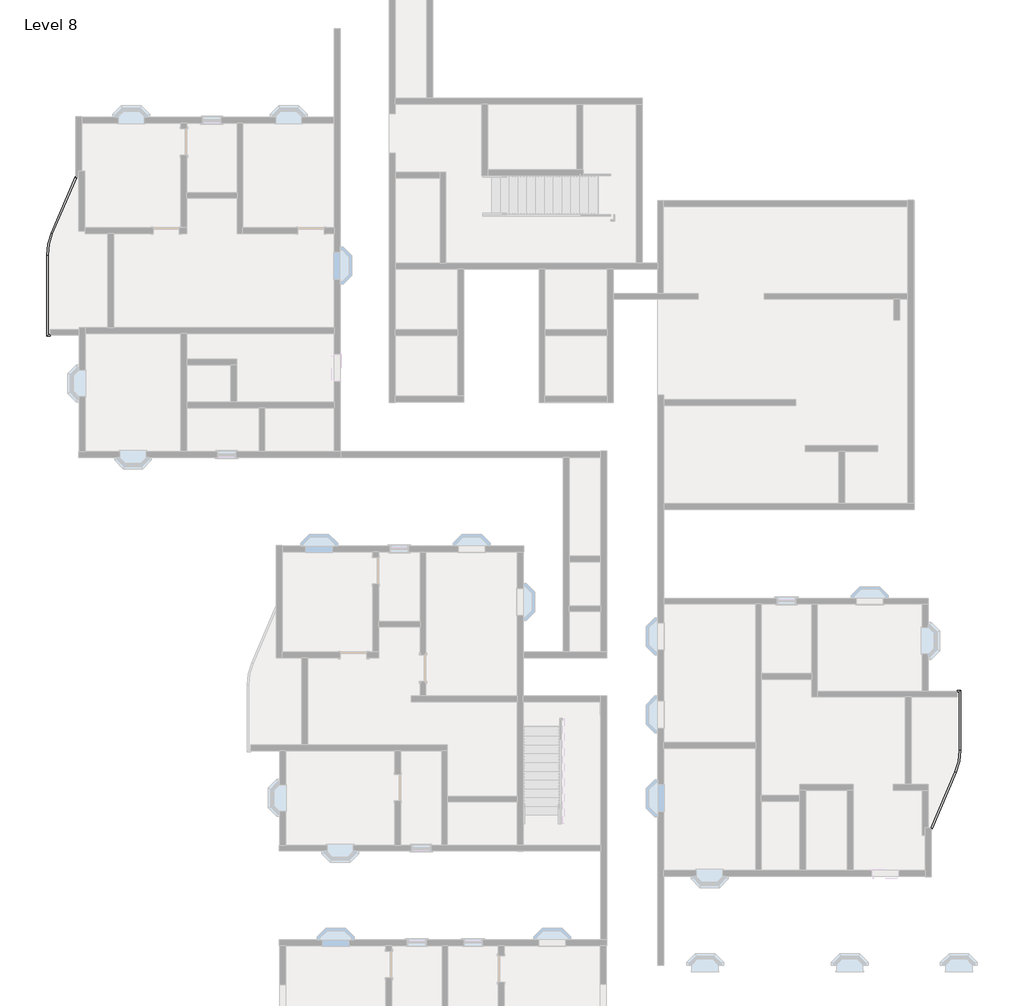
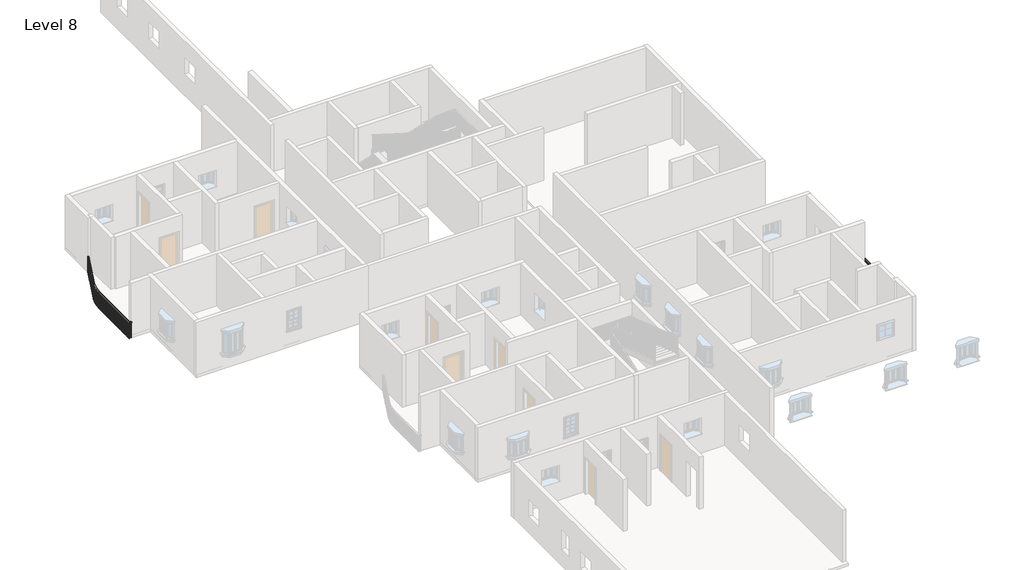
# One storey, part 9 of 14: 2 railings.
"""IFC4 building model written with IfcOpenShell, lengths in millimetres."""

from ifc_helpers import new_model, si_unit, frame, origin, place, context, project, spatial, polyline, circle_curve, outline, extrude, element, save
from ifc_brep_helpers import plane_surface, cylinder_surface, revolved_surface, advanced_brep

model = new_model("IFC4")

# Units and contexts
model_context = context("Model", 3, world=origin())
ifc_project = project(units=[si_unit("LENGTHUNIT", "METRE", prefix="MILLI")], contexts=[model_context])

# Site, building, storey
site = spatial("IfcSite", under=ifc_project)
building = spatial("IfcBuilding", under=site)
storey = spatial("IfcBuildingStorey", under=building, Name="Level 8", Elevation=21336.0)

# Railings
placement = place(None, origin())
element("IfcRailing", 1, ObjectType="Handrail - Rectangular", at=placement, inside=storey, context=model_context, shape_type="SolidModel", body=[
    advanced_brep(
    [(-19327.739878, 12446.0257339, 22250.4), (-19327.739878, 12446.0257339, 22199.6), (-19374.4383922, 12466.022953, 22199.6), (-19374.4383922, 12466.022953, 22250.4), (-20162.483418, 10496.6905323, 22250.4), (-20162.483418, 10496.6905323, 22199.6), (-20209.1819322, 10516.6877514, 22199.6), (-20209.1819322, 10516.6877514, 22250.4), (-20316.2891351, 9746.7948172, 22199.6), (-20316.2891351, 9746.7948172, 22250.4), (-20367.0891351, 9746.7948172, 22199.6), (-20367.0891351, 9746.7948172, 22250.4), (-20316.2891351, 7005.2583494, 22250.4), (-20316.2891351, 7005.2583494, 22199.6), (-20367.0891351, 6954.4583494, 22199.6), (-20367.0891351, 6954.4583494, 22250.4), (-20240.0891351, 7005.2583494, 22250.4), (-20240.0891351, 6954.4583494, 22250.4), (-20240.0891351, 6954.4583494, 22199.6), (-20240.0891351, 7005.2583494, 22199.6)],
    [
        (0, 1),
        (1, 2),
        (2, 3),
        (3, 0),
        (0, 4),
        (4, 5),
        (5, 1),
        (5, 6),
        (6, 2),
        (6, 7),
        (7, 3),
        (7, 4),
        (8, 5, circle_curve(frame((-18411.2891351, 9746.7948172, 22199.6), z_axis=(0.0, 0.0, -1.0), x_axis=(-0.919262090762392, 0.3936460446735823, 0.0)), 1905.0)),
        (4, 9, circle_curve(frame((-18411.2891351, 9746.7948172, 22250.4), z_axis=(0.0, 0.0, 1.0), x_axis=(-0.919262090762392, 0.3936460446735823, 0.0)), 1905.0)),
        (9, 8),
        (10, 6, circle_curve(frame((-18411.2891351, 9746.7948172, 22199.6), z_axis=(0.0, 0.0, -1.0), x_axis=(-0.919262090762392, 0.3936460446735823, 0.0)), 1955.8)),
        (8, 10),
        (11, 7, circle_curve(frame((-18411.2891351, 9746.7948172, 22250.4), z_axis=(0.0, 0.0, -1.0), x_axis=(-0.919262090762392, 0.3936460446735823, 0.0)), 1955.8)),
        (10, 11),
        (11, 9),
        (9, 12),
        (12, 13),
        (13, 8),
        (13, 14),
        (14, 10),
        (14, 15),
        (15, 11),
        (15, 12),
        (16, 17),
        (17, 18),
        (18, 19),
        (19, 16),
        (12, 16),
        (19, 13),
        (18, 14),
        (17, 15),
    ],
    [
        plane_surface(frame((-19351.0891351, 12456.0243434, 22250.4), z_axis=(0.3936460446735829, 0.9192620907623917, 0.0), x_axis=(0.9192620907623917, -0.3936460446735829, 0.0))),
        plane_surface(frame((-19327.739878, 12446.0257339, 22250.4), z_axis=(0.9192620907623916, -0.393646044673583, 0.0), x_axis=(-0.393646044673583, -0.9192620907623916, 0.0))),
        plane_surface(frame((-19327.739878, 12446.0257339, 22199.6), z_axis=(0.0, 0.0, -1.0), x_axis=(-0.393646044673583, -0.9192620907623916, 0.0))),
        plane_surface(frame((-19374.4383922, 12466.022953, 22199.6), z_axis=(-0.9192620907623917, 0.3936460446735826, 0.0), x_axis=(-0.3936460446735826, -0.9192620907623917, 0.0))),
        plane_surface(frame((-19374.4383922, 12466.022953, 22250.4), z_axis=(0.0, 0.0, 1.0), x_axis=(-0.3936460446735826, -0.9192620907623917, 0.0))),
        revolved_surface(polyline([(-20162.483418002357, 10496.690532303173, 22250.4), (-20162.483418002357, 10496.690532303173, 22199.6)]), (-18411.2891351, 9746.7948172, 22250.4), (0.0, 0.0, 1.0)),
        plane_surface(frame((-18411.2891351, 9746.7948172, 22199.6), z_axis=(0.0, 0.0, -1.0), x_axis=(-0.919262090762392, 0.3936460446735823, 0.0))),
        cylinder_surface(frame((-18411.2891351, 9746.7948172, 22250.4), z_axis=(0.0, 0.0, 1.0), x_axis=(-0.919262090762392, 0.3936460446735823, 0.0)), 1955.8),
        plane_surface(frame((-18411.2891351, 9746.7948172, 22250.4), z_axis=(0.0, 0.0, 1.0), x_axis=(-0.919262090762392, 0.3936460446735823, 0.0))),
        plane_surface(frame((-20316.2891351, 9746.7948172, 22250.4), z_axis=(1.0, 0.0, 0.0), x_axis=(0.0, -1.0, 0.0))),
        plane_surface(frame((-20316.2891351, 9746.7948172, 22199.6), z_axis=(0.0, 0.0, -1.0), x_axis=(0.0, -1.0, 0.0))),
        plane_surface(frame((-20367.0891351, 9746.7948172, 22199.6), z_axis=(-1.0, 0.0, 0.0), x_axis=(0.0, -1.0, 0.0))),
        plane_surface(frame((-20367.0891351, 9746.7948172, 22250.4), z_axis=(0.0, 0.0, 1.0), x_axis=(0.0, -1.0, 0.0))),
        plane_surface(frame((-20240.0891351, 6979.8583494, 22250.4), z_axis=(1.0, 0.0, 0.0), x_axis=(0.0, 1.0, 0.0))),
        plane_surface(frame((-20316.2891351, 7005.2583494, 22250.4), z_axis=(0.0, 1.0, 0.0), x_axis=(1.0, 0.0, 0.0))),
        plane_surface(frame((-20316.2891351, 7005.2583494, 22199.6), z_axis=(0.0, 0.0, -1.0), x_axis=(1.0, 0.0, 0.0))),
        plane_surface(frame((-20367.0891351, 6954.4583494, 22199.6), z_axis=(0.0, -1.0, 0.0), x_axis=(1.0, 0.0, 0.0))),
        plane_surface(frame((-20367.0891351, 6954.4583494, 22250.4), z_axis=(0.0, 0.0, 1.0), x_axis=(1.0, 0.0, 0.0))),
    ],
    [
        (0, [[1, 2, 3, 4]]),
        (1, [[-1, 5, 6, 7]]),
        (2, [[-2, -7, 8, 9]]),
        (3, [[-3, -9, 10, 11]]),
        (4, [[-4, -11, 12, -5]]),
        (5, [[13, -6, 14, 15]]),
        (6, [[16, -8, -13, 17]]),
        (7, [[18, -10, -16, 19]]),
        (8, [[-14, -12, -18, 20]]),
        (9, [[-15, 21, 22, 23]]),
        (10, [[-17, -23, 24, 25]]),
        (11, [[-19, -25, 26, 27]]),
        (12, [[-20, -27, 28, -21]]),
        (13, [[29, 30, 31, 32]]),
        (14, [[-22, 33, -32, 34]]),
        (15, [[-24, -34, -31, 35]]),
        (16, [[-26, -35, -30, 36]]),
        (17, [[-28, -36, -29, -33]]),
    ],
),
    extrude(outline(polyline([(-20351.2141351, 7013.1198172), (-20332.1641351, 7013.1198172), (-20332.1641351, 6994.0698172), (-20351.2141351, 6994.0698172), (-20351.2141351, 7013.1198172)])), frame((0.0, 0.0, 21336.0), z_axis=(0.0, 0.0, 1.0), x_axis=(1.0, 0.0, 0.0)), (0.0, 0.0, 1.0), 863.6),
    extrude(outline(polyline([(-20351.2141351, 7114.7198172), (-20332.1641351, 7114.7198172), (-20332.1641351, 7095.6698172), (-20351.2141351, 7095.6698172), (-20351.2141351, 7114.7198172)])), frame((0.0, 0.0, 21336.0), z_axis=(0.0, 0.0, 1.0), x_axis=(1.0, 0.0, 0.0)), (0.0, 0.0, 1.0), 863.6),
    extrude(outline(polyline([(-20351.2141351, 7216.3198172), (-20332.1641351, 7216.3198172), (-20332.1641351, 7197.2698172), (-20351.2141351, 7197.2698172), (-20351.2141351, 7216.3198172)])), frame((0.0, 0.0, 21336.0), z_axis=(0.0, 0.0, 1.0), x_axis=(1.0, 0.0, 0.0)), (0.0, 0.0, 1.0), 863.6),
    extrude(outline(polyline([(-20351.2141351, 7317.9198172), (-20332.1641351, 7317.9198172), (-20332.1641351, 7298.8698172), (-20351.2141351, 7298.8698172), (-20351.2141351, 7317.9198172)])), frame((0.0, 0.0, 21336.0), z_axis=(0.0, 0.0, 1.0), x_axis=(1.0, 0.0, 0.0)), (0.0, 0.0, 1.0), 863.6),
    extrude(outline(polyline([(-20351.2141351, 7419.5198172), (-20332.1641351, 7419.5198172), (-20332.1641351, 7400.4698172), (-20351.2141351, 7400.4698172), (-20351.2141351, 7419.5198172)])), frame((0.0, 0.0, 21336.0), z_axis=(0.0, 0.0, 1.0), x_axis=(1.0, 0.0, 0.0)), (0.0, 0.0, 1.0), 863.6),
    extrude(outline(polyline([(-20351.2141351, 7521.1198172), (-20332.1641351, 7521.1198172), (-20332.1641351, 7502.0698172), (-20351.2141351, 7502.0698172), (-20351.2141351, 7521.1198172)])), frame((0.0, 0.0, 21336.0), z_axis=(0.0, 0.0, 1.0), x_axis=(1.0, 0.0, 0.0)), (0.0, 0.0, 1.0), 863.6),
    extrude(outline(polyline([(-20351.2141351, 7622.7198172), (-20332.1641351, 7622.7198172), (-20332.1641351, 7603.6698172), (-20351.2141351, 7603.6698172), (-20351.2141351, 7622.7198172)])), frame((0.0, 0.0, 21336.0), z_axis=(0.0, 0.0, 1.0), x_axis=(1.0, 0.0, 0.0)), (0.0, 0.0, 1.0), 863.6),
    extrude(outline(polyline([(-20351.2141351, 7724.3198172), (-20332.1641351, 7724.3198172), (-20332.1641351, 7705.2698172), (-20351.2141351, 7705.2698172), (-20351.2141351, 7724.3198172)])), frame((0.0, 0.0, 21336.0), z_axis=(0.0, 0.0, 1.0), x_axis=(1.0, 0.0, 0.0)), (0.0, 0.0, 1.0), 863.6),
    extrude(outline(polyline([(-20351.2141351, 7825.9198172), (-20332.1641351, 7825.9198172), (-20332.1641351, 7806.8698172), (-20351.2141351, 7806.8698172), (-20351.2141351, 7825.9198172)])), frame((0.0, 0.0, 21336.0), z_axis=(0.0, 0.0, 1.0), x_axis=(1.0, 0.0, 0.0)), (0.0, 0.0, 1.0), 863.6),
    extrude(outline(polyline([(-20351.2141351, 7927.5198172), (-20332.1641351, 7927.5198172), (-20332.1641351, 7908.4698172), (-20351.2141351, 7908.4698172), (-20351.2141351, 7927.5198172)])), frame((0.0, 0.0, 21336.0), z_axis=(0.0, 0.0, 1.0), x_axis=(1.0, 0.0, 0.0)), (0.0, 0.0, 1.0), 863.6),
    extrude(outline(polyline([(-20351.2141351, 8029.1198172), (-20332.1641351, 8029.1198172), (-20332.1641351, 8010.0698172), (-20351.2141351, 8010.0698172), (-20351.2141351, 8029.1198172)])), frame((0.0, 0.0, 21336.0), z_axis=(0.0, 0.0, 1.0), x_axis=(1.0, 0.0, 0.0)), (0.0, 0.0, 1.0), 863.6),
    extrude(outline(polyline([(-20351.2141351, 8130.7198172), (-20332.1641351, 8130.7198172), (-20332.1641351, 8111.6698172), (-20351.2141351, 8111.6698172), (-20351.2141351, 8130.7198172)])), frame((0.0, 0.0, 21336.0), z_axis=(0.0, 0.0, 1.0), x_axis=(1.0, 0.0, 0.0)), (0.0, 0.0, 1.0), 863.6),
    extrude(outline(polyline([(-20351.2141351, 8232.3198172), (-20332.1641351, 8232.3198172), (-20332.1641351, 8213.2698172), (-20351.2141351, 8213.2698172), (-20351.2141351, 8232.3198172)])), frame((0.0, 0.0, 21336.0), z_axis=(0.0, 0.0, 1.0), x_axis=(1.0, 0.0, 0.0)), (0.0, 0.0, 1.0), 863.6),
    extrude(outline(polyline([(-20351.2141351, 8333.9198172), (-20332.1641351, 8333.9198172), (-20332.1641351, 8314.8698172), (-20351.2141351, 8314.8698172), (-20351.2141351, 8333.9198172)])), frame((0.0, 0.0, 21336.0), z_axis=(0.0, 0.0, 1.0), x_axis=(1.0, 0.0, 0.0)), (0.0, 0.0, 1.0), 863.6),
    extrude(outline(polyline([(-20351.2141351, 8435.5198172), (-20332.1641351, 8435.5198172), (-20332.1641351, 8416.4698172), (-20351.2141351, 8416.4698172), (-20351.2141351, 8435.5198172)])), frame((0.0, 0.0, 21336.0), z_axis=(0.0, 0.0, 1.0), x_axis=(1.0, 0.0, 0.0)), (0.0, 0.0, 1.0), 863.6),
    extrude(outline(polyline([(-20351.2141351, 8537.1198172), (-20332.1641351, 8537.1198172), (-20332.1641351, 8518.0698172), (-20351.2141351, 8518.0698172), (-20351.2141351, 8537.1198172)])), frame((0.0, 0.0, 21336.0), z_axis=(0.0, 0.0, 1.0), x_axis=(1.0, 0.0, 0.0)), (0.0, 0.0, 1.0), 863.6),
    extrude(outline(polyline([(-20351.2141351, 8638.7198172), (-20332.1641351, 8638.7198172), (-20332.1641351, 8619.6698172), (-20351.2141351, 8619.6698172), (-20351.2141351, 8638.7198172)])), frame((0.0, 0.0, 21336.0), z_axis=(0.0, 0.0, 1.0), x_axis=(1.0, 0.0, 0.0)), (0.0, 0.0, 1.0), 863.6),
    extrude(outline(polyline([(-20351.2141351, 8740.3198172), (-20332.1641351, 8740.3198172), (-20332.1641351, 8721.2698172), (-20351.2141351, 8721.2698172), (-20351.2141351, 8740.3198172)])), frame((0.0, 0.0, 21336.0), z_axis=(0.0, 0.0, 1.0), x_axis=(1.0, 0.0, 0.0)), (0.0, 0.0, 1.0), 863.6),
    extrude(outline(polyline([(-20351.2141351, 8841.9198172), (-20332.1641351, 8841.9198172), (-20332.1641351, 8822.8698172), (-20351.2141351, 8822.8698172), (-20351.2141351, 8841.9198172)])), frame((0.0, 0.0, 21336.0), z_axis=(0.0, 0.0, 1.0), x_axis=(1.0, 0.0, 0.0)), (0.0, 0.0, 1.0), 863.6),
    extrude(outline(polyline([(-20351.2141351, 8943.5198172), (-20332.1641351, 8943.5198172), (-20332.1641351, 8924.4698172), (-20351.2141351, 8924.4698172), (-20351.2141351, 8943.5198172)])), frame((0.0, 0.0, 21336.0), z_axis=(0.0, 0.0, 1.0), x_axis=(1.0, 0.0, 0.0)), (0.0, 0.0, 1.0), 863.6),
    extrude(outline(polyline([(-20351.2141351, 9045.1198172), (-20332.1641351, 9045.1198172), (-20332.1641351, 9026.0698172), (-20351.2141351, 9026.0698172), (-20351.2141351, 9045.1198172)])), frame((0.0, 0.0, 21336.0), z_axis=(0.0, 0.0, 1.0), x_axis=(1.0, 0.0, 0.0)), (0.0, 0.0, 1.0), 863.6),
    extrude(outline(polyline([(-20351.2141351, 9146.7198172), (-20332.1641351, 9146.7198172), (-20332.1641351, 9127.6698172), (-20351.2141351, 9127.6698172), (-20351.2141351, 9146.7198172)])), frame((0.0, 0.0, 21336.0), z_axis=(0.0, 0.0, 1.0), x_axis=(1.0, 0.0, 0.0)), (0.0, 0.0, 1.0), 863.6),
    extrude(outline(polyline([(-20351.2141351, 9248.3198172), (-20332.1641351, 9248.3198172), (-20332.1641351, 9229.2698172), (-20351.2141351, 9229.2698172), (-20351.2141351, 9248.3198172)])), frame((0.0, 0.0, 21336.0), z_axis=(0.0, 0.0, 1.0), x_axis=(1.0, 0.0, 0.0)), (0.0, 0.0, 1.0), 863.6),
    extrude(outline(polyline([(-20351.2141351, 9349.9198172), (-20332.1641351, 9349.9198172), (-20332.1641351, 9330.8698172), (-20351.2141351, 9330.8698172), (-20351.2141351, 9349.9198172)])), frame((0.0, 0.0, 21336.0), z_axis=(0.0, 0.0, 1.0), x_axis=(1.0, 0.0, 0.0)), (0.0, 0.0, 1.0), 863.6),
    extrude(outline(polyline([(-20351.2141351, 9451.5198172), (-20332.1641351, 9451.5198172), (-20332.1641351, 9432.4698172), (-20351.2141351, 9432.4698172), (-20351.2141351, 9451.5198172)])), frame((0.0, 0.0, 21336.0), z_axis=(0.0, 0.0, 1.0), x_axis=(1.0, 0.0, 0.0)), (0.0, 0.0, 1.0), 863.6),
    extrude(outline(polyline([(-20351.2141351, 9553.1198172), (-20332.1641351, 9553.1198172), (-20332.1641351, 9534.0698172), (-20351.2141351, 9534.0698172), (-20351.2141351, 9553.1198172)])), frame((0.0, 0.0, 21336.0), z_axis=(0.0, 0.0, 1.0), x_axis=(1.0, 0.0, 0.0)), (0.0, 0.0, 1.0), 863.6),
    extrude(outline(polyline([(-20351.2141351, 9654.7198172), (-20332.1641351, 9654.7198172), (-20332.1641351, 9635.6698172), (-20351.2141351, 9635.6698172), (-20351.2141351, 9654.7198172)])), frame((0.0, 0.0, 21336.0), z_axis=(0.0, 0.0, 1.0), x_axis=(1.0, 0.0, 0.0)), (0.0, 0.0, 1.0), 863.6),
    extrude(outline(polyline([(-20349.6005818, 9826.4720848), (-20330.5630441, 9825.7831307), (-20331.2519982, 9806.745593), (-20350.289536, 9807.4345471), (-20349.6005818, 9826.4720848)])), frame((0.0, 0.0, 21336.0), z_axis=(0.0, 0.0, 1.0), x_axis=(1.0, 0.0, 0.0)), (0.0, 0.0, 1.0), 863.6),
    extrude(outline(polyline([(-20342.724955, 9928.3310534), (-20323.750023, 9926.6415402), (-20325.4395363, 9907.6666081), (-20344.4144683, 9909.3561214), (-20342.724955, 9928.3310534)])), frame((0.0, 0.0, 21336.0), z_axis=(0.0, 0.0, 1.0), x_axis=(1.0, 0.0, 0.0)), (0.0, 0.0, 1.0), 863.6),
    extrude(outline(polyline([(-20330.5003254, 10029.6872677), (-20311.6405491, 10027.0018743), (-20314.3259425, 10008.142098), (-20333.1857188, 10010.8274914), (-20330.5003254, 10029.6872677)])), frame((0.0, 0.0, 21336.0), z_axis=(0.0, 0.0, 1.0), x_axis=(1.0, 0.0, 0.0)), (0.0, 0.0, 1.0), 863.6),
    extrude(outline(polyline([(-20312.9605484, 10130.2600272), (-20294.2681589, 10126.5861907), (-20297.9419954, 10107.8938012), (-20316.6343849, 10111.5676377), (-20312.9605484, 10130.2600272)])), frame((0.0, 0.0, 21336.0), z_axis=(0.0, 0.0, 1.0), x_axis=(1.0, 0.0, 0.0)), (0.0, 0.0, 1.0), 863.6),
    extrude(outline(polyline([(-20290.1541995, 10229.7708014), (-20271.6809643, 10225.1186963), (-20276.3330693, 10206.6454611), (-20294.8063045, 10211.2975662), (-20290.1541995, 10229.7708014)])), frame((0.0, 0.0, 21336.0), z_axis=(0.0, 0.0, 1.0), x_axis=(1.0, 0.0, 0.0)), (0.0, 0.0, 1.0), 863.6),
    extrude(outline(polyline([(-20262.1444395, 10327.9440008), (-20243.9415192, 10322.3265109), (-20249.5590091, 10304.1235906), (-20267.7619294, 10309.7410805), (-20262.1444395, 10327.9440008)])), frame((0.0, 0.0, 21336.0), z_axis=(0.0, 0.0, 1.0), x_axis=(1.0, 0.0, 0.0)), (0.0, 0.0, 1.0), 863.6),
    extrude(outline(polyline([(-20229.0088399, 10424.5077402), (-20211.1266465, 10417.9404228), (-20217.693964, 10400.0582293), (-20235.5761574, 10406.6255468), (-20229.0088399, 10424.5077402)])), frame((0.0, 0.0, 21336.0), z_axis=(0.0, 0.0, 1.0), x_axis=(1.0, 0.0, 0.0)), (0.0, 0.0, 1.0), 863.6),
    extrude(outline(polyline([(-20155.9843907, 10600.589225), (-20138.4724479, 10593.0902678), (-20145.9714051, 10575.578325), (-20163.4833479, 10583.0772822), (-20155.9843907, 10600.589225)])), frame((0.0, 0.0, 21336.0), z_axis=(0.0, 0.0, 1.0), x_axis=(1.0, 0.0, 0.0)), (0.0, 0.0, 1.0), 863.6),
    extrude(outline(polyline([(-20115.9899526, 10693.9862534), (-20098.4780098, 10686.4872963), (-20105.9769669, 10668.9753534), (-20123.4889098, 10676.4743106), (-20115.9899526, 10693.9862534)])), frame((0.0, 0.0, 21336.0), z_axis=(0.0, 0.0, 1.0), x_axis=(1.0, 0.0, 0.0)), (0.0, 0.0, 1.0), 863.6),
    extrude(outline(polyline([(-20075.9955145, 10787.3832818), (-20058.4835716, 10779.8843247), (-20065.9825288, 10762.3723818), (-20083.4944716, 10769.871339), (-20075.9955145, 10787.3832818)])), frame((0.0, 0.0, 21336.0), z_axis=(0.0, 0.0, 1.0), x_axis=(1.0, 0.0, 0.0)), (0.0, 0.0, 1.0), 863.6),
    extrude(outline(polyline([(-20036.0010763, 10880.7803103), (-20018.4891335, 10873.2813531), (-20025.9880906, 10855.7694103), (-20043.5000335, 10863.2683674), (-20036.0010763, 10880.7803103)])), frame((0.0, 0.0, 21336.0), z_axis=(0.0, 0.0, 1.0), x_axis=(1.0, 0.0, 0.0)), (0.0, 0.0, 1.0), 863.6),
    extrude(outline(polyline([(-19996.0066382, 10974.1773387), (-19978.4946954, 10966.6783815), (-19985.9936525, 10949.1664387), (-20003.5055953, 10956.6653958), (-19996.0066382, 10974.1773387)])), frame((0.0, 0.0, 21336.0), z_axis=(0.0, 0.0, 1.0), x_axis=(1.0, 0.0, 0.0)), (0.0, 0.0, 1.0), 863.6),
    extrude(outline(polyline([(-19956.0122, 11067.5743671), (-19938.5002572, 11060.0754099), (-19945.9992144, 11042.5634671), (-19963.5111572, 11050.0624243), (-19956.0122, 11067.5743671)])), frame((0.0, 0.0, 21336.0), z_axis=(0.0, 0.0, 1.0), x_axis=(1.0, 0.0, 0.0)), (0.0, 0.0, 1.0), 863.6),
    extrude(outline(polyline([(-19916.0177619, 11160.9713955), (-19898.5058191, 11153.4724384), (-19906.0047762, 11135.9604955), (-19923.5167191, 11143.4594527), (-19916.0177619, 11160.9713955)])), frame((0.0, 0.0, 21336.0), z_axis=(0.0, 0.0, 1.0), x_axis=(1.0, 0.0, 0.0)), (0.0, 0.0, 1.0), 863.6),
    extrude(outline(polyline([(-19876.0233238, 11254.3684239), (-19858.5113809, 11246.8694668), (-19866.0103381, 11229.357524), (-19883.5222809, 11236.8564811), (-19876.0233238, 11254.3684239)])), frame((0.0, 0.0, 21336.0), z_axis=(0.0, 0.0, 1.0), x_axis=(1.0, 0.0, 0.0)), (0.0, 0.0, 1.0), 863.6),
    extrude(outline(polyline([(-19836.0288856, 11347.7654524), (-19818.5169428, 11340.2664952), (-19826.0159, 11322.7545524), (-19843.5278428, 11330.2535095), (-19836.0288856, 11347.7654524)])), frame((0.0, 0.0, 21336.0), z_axis=(0.0, 0.0, 1.0), x_axis=(1.0, 0.0, 0.0)), (0.0, 0.0, 1.0), 863.6),
    extrude(outline(polyline([(-19796.0344475, 11441.1624808), (-19778.5225047, 11433.6635236), (-19786.0214618, 11416.1515808), (-19803.5334046, 11423.650538), (-19796.0344475, 11441.1624808)])), frame((0.0, 0.0, 21336.0), z_axis=(0.0, 0.0, 1.0), x_axis=(1.0, 0.0, 0.0)), (0.0, 0.0, 1.0), 863.6),
    extrude(outline(polyline([(-19756.0400094, 11534.5595092), (-19738.5280665, 11527.060552), (-19746.0270237, 11509.5486092), (-19763.5389665, 11517.0475664), (-19756.0400094, 11534.5595092)])), frame((0.0, 0.0, 21336.0), z_axis=(0.0, 0.0, 1.0), x_axis=(1.0, 0.0, 0.0)), (0.0, 0.0, 1.0), 863.6),
    extrude(outline(polyline([(-19716.0455712, 11627.9565376), (-19698.5336284, 11620.4575805), (-19706.0325855, 11602.9456376), (-19723.5445284, 11610.4445948), (-19716.0455712, 11627.9565376)])), frame((0.0, 0.0, 21336.0), z_axis=(0.0, 0.0, 1.0), x_axis=(1.0, 0.0, 0.0)), (0.0, 0.0, 1.0), 863.6),
    extrude(outline(polyline([(-19676.0511331, 11721.353566), (-19658.5391902, 11713.8546089), (-19666.0381474, 11696.3426661), (-19683.5500902, 11703.8416232), (-19676.0511331, 11721.353566)])), frame((0.0, 0.0, 21336.0), z_axis=(0.0, 0.0, 1.0), x_axis=(1.0, 0.0, 0.0)), (0.0, 0.0, 1.0), 863.6),
    extrude(outline(polyline([(-19636.0566949, 11814.7505945), (-19618.5447521, 11807.2516373), (-19626.0437093, 11789.7396945), (-19643.5556521, 11797.2386516), (-19636.0566949, 11814.7505945)])), frame((0.0, 0.0, 21336.0), z_axis=(0.0, 0.0, 1.0), x_axis=(1.0, 0.0, 0.0)), (0.0, 0.0, 1.0), 863.6),
    extrude(outline(polyline([(-19596.0622568, 11908.1476229), (-19578.550314, 11900.6486657), (-19586.0492711, 11883.1367229), (-19603.561214, 11890.6356801), (-19596.0622568, 11908.1476229)])), frame((0.0, 0.0, 21336.0), z_axis=(0.0, 0.0, 1.0), x_axis=(1.0, 0.0, 0.0)), (0.0, 0.0, 1.0), 863.6),
    extrude(outline(polyline([(-19556.0678187, 12001.5446513), (-19538.5558758, 11994.0456942), (-19546.054833, 11976.5337513), (-19563.5667758, 11984.0327085), (-19556.0678187, 12001.5446513)])), frame((0.0, 0.0, 21336.0), z_axis=(0.0, 0.0, 1.0), x_axis=(1.0, 0.0, 0.0)), (0.0, 0.0, 1.0), 863.6),
    extrude(outline(polyline([(-19516.0733805, 12094.9416797), (-19498.5614377, 12087.4427226), (-19506.0603948, 12069.9307797), (-19523.5723377, 12077.4297369), (-19516.0733805, 12094.9416797)])), frame((0.0, 0.0, 21336.0), z_axis=(0.0, 0.0, 1.0), x_axis=(1.0, 0.0, 0.0)), (0.0, 0.0, 1.0), 863.6),
    extrude(outline(polyline([(-19476.0789424, 12188.3387082), (-19458.5669996, 12180.839751), (-19466.0659567, 12163.3278082), (-19483.5778995, 12170.8267653), (-19476.0789424, 12188.3387082)])), frame((0.0, 0.0, 21336.0), z_axis=(0.0, 0.0, 1.0), x_axis=(1.0, 0.0, 0.0)), (0.0, 0.0, 1.0), 863.6),
    extrude(outline(polyline([(-19436.0845042, 12281.7357366), (-19418.5725614, 12274.2367794), (-19426.0715186, 12256.7248366), (-19443.5834614, 12264.2237937), (-19436.0845042, 12281.7357366)])), frame((0.0, 0.0, 21336.0), z_axis=(0.0, 0.0, 1.0), x_axis=(1.0, 0.0, 0.0)), (0.0, 0.0, 1.0), 863.6),
    extrude(outline(polyline([(-19396.0900661, 12375.132765), (-19378.5781233, 12367.6338078), (-19386.0770804, 12350.121865), (-19403.5890233, 12357.6208222), (-19396.0900661, 12375.132765)])), frame((0.0, 0.0, 21336.0), z_axis=(0.0, 0.0, 1.0), x_axis=(1.0, 0.0, 0.0)), (0.0, 0.0, 1.0), 863.6),
    extrude(outline(polyline([(-20351.2141351, 6989.3833494), (-20332.1641351, 6989.3833494), (-20332.1641351, 6970.3333494), (-20351.2141351, 6970.3333494), (-20351.2141351, 6989.3833494)])), frame((0.0, 0.0, 21336.0), z_axis=(0.0, 0.0, 1.0), x_axis=(1.0, 0.0, 0.0)), (0.0, 0.0, 1.0), 863.6),
    extrude(outline(polyline([(-20351.2141351, 9756.3198172), (-20332.1641351, 9756.3198172), (-20332.1641351, 9737.2698172), (-20351.2141351, 9737.2698172), (-20351.2141351, 9756.3198172)])), frame((0.0, 0.0, 21336.0), z_axis=(0.0, 0.0, 1.0), x_axis=(1.0, 0.0, 0.0)), (0.0, 0.0, 1.0), 863.6),
    extrude(outline(polyline([(-20190.839168, 10519.1945919), (-20173.3272251, 10511.6956347), (-20180.8261823, 10494.1836919), (-20198.3381251, 10501.682649), (-20190.839168, 10519.1945919)])), frame((0.0, 0.0, 21336.0), z_axis=(0.0, 0.0, 1.0), x_axis=(1.0, 0.0, 0.0)), (0.0, 0.0, 1.0), 863.6),
    extrude(outline(polyline([(-20259.1391351, 6970.3333494), (-20259.1391351, 6989.3833494), (-20240.0891351, 6989.3833494), (-20240.0891351, 6970.3333494), (-20259.1391351, 6970.3333494)])), frame((0.0, 0.0, 21336.0), z_axis=(0.0, 0.0, 1.0), x_axis=(1.0, 0.0, 0.0)), (0.0, 0.0, 1.0), 863.6),
    extrude(outline(polyline([(-19359.8451065, 12459.773822), (-19342.3331637, 12452.2748648), (-19349.8321209, 12434.762922), (-19367.3440637, 12442.2618792), (-19359.8451065, 12459.773822)])), frame((0.0, 0.0, 21336.0), z_axis=(0.0, 0.0, 1.0), x_axis=(1.0, 0.0, 0.0)), (0.0, 0.0, 1.0), 863.6),
])
element("IfcRailing", 2, ObjectType="Handrail - Rectangular", at=placement, inside=storey, context=model_context, shape_type="SolidModel", body=[
    advanced_brep(
    [(10250.7887952, -10096.81198, 22250.4), (10250.7887952, -10096.81198, 22199.6), (10297.4873094, -10116.8091991, 22199.6), (10297.4873094, -10116.8091991, 22250.4), (11085.5323352, -8147.4767784, 22250.4), (11085.5323352, -8147.4767784, 22199.6), (11132.2308494, -8167.4739975, 22199.6), (11132.2308494, -8167.4739975, 22250.4), (11239.3380523, -7397.5810633, 22199.6), (11239.3380523, -7397.5810633, 22250.4), (11290.1380523, -7397.5810633, 22199.6), (11290.1380523, -7397.5810633, 22250.4), (11239.3380523, -5378.0542694, 22250.4), (11239.3380523, -5378.0542694, 22199.6), (11290.1380523, -5327.2542694, 22199.6), (11290.1380523, -5327.2542694, 22250.4), (11163.1380523, -5378.0542694, 22250.4), (11163.1380523, -5327.2542694, 22250.4), (11163.1380523, -5327.2542694, 22199.6), (11163.1380523, -5378.0542694, 22199.6)],
    [
        (0, 1),
        (1, 2),
        (2, 3),
        (3, 0),
        (0, 4),
        (4, 5),
        (5, 1),
        (5, 6),
        (6, 2),
        (6, 7),
        (7, 3),
        (7, 4),
        (8, 5, circle_curve(frame((9334.3380523, -7397.5810633, 22199.6), z_axis=(0.0, 0.0, -1.0), x_axis=(0.9192620907624003, -0.3936460446735628, 0.0)), 1905.0)),
        (4, 9, circle_curve(frame((9334.3380523, -7397.5810633, 22250.4), z_axis=(0.0, 0.0, 1.0), x_axis=(0.9192620907624003, -0.3936460446735628, 0.0)), 1905.0)),
        (9, 8),
        (10, 6, circle_curve(frame((9334.3380523, -7397.5810633, 22199.6), z_axis=(0.0, 0.0, -1.0), x_axis=(0.9192620907624003, -0.3936460446735628, 0.0)), 1955.8)),
        (8, 10),
        (11, 7, circle_curve(frame((9334.3380523, -7397.5810633, 22250.4), z_axis=(0.0, 0.0, -1.0), x_axis=(0.9192620907624003, -0.3936460446735628, 0.0)), 1955.8)),
        (10, 11),
        (11, 9),
        (9, 12),
        (12, 13),
        (13, 8),
        (13, 14),
        (14, 10),
        (14, 15),
        (15, 11),
        (15, 12),
        (16, 17),
        (17, 18),
        (18, 19),
        (19, 16),
        (12, 16),
        (19, 13),
        (18, 14),
        (17, 15),
    ],
    [
        plane_surface(frame((10274.1380523, -10106.8105895, 22250.4), z_axis=(-0.3936460446735629, -0.9192620907624003, 0.0), x_axis=(0.9192620907624003, -0.3936460446735629, 0.0))),
        plane_surface(frame((10250.7887952, -10096.81198, 22250.4), z_axis=(-0.9192620907624003, 0.3936460446735627, 0.0), x_axis=(0.3936460446735627, 0.9192620907624003, 0.0))),
        plane_surface(frame((10250.7887952, -10096.81198, 22199.6), z_axis=(0.0, 0.0, -1.0), x_axis=(0.3936460446735627, 0.9192620907624003, 0.0))),
        plane_surface(frame((10297.4873094, -10116.8091991, 22199.6), z_axis=(0.9192620907624003, -0.3936460446735629, 0.0), x_axis=(0.3936460446735629, 0.9192620907624003, 0.0))),
        plane_surface(frame((10297.4873094, -10116.8091991, 22250.4), z_axis=(0.0, 0.0, 1.0), x_axis=(0.3936460446735629, 0.9192620907624003, 0.0))),
        revolved_surface(polyline([(11085.532335202372, -8147.476778403137, 22250.4), (11085.532335202372, -8147.476778403137, 22199.6)]), (9334.3380523, -7397.5810633, 22250.4), (0.0, 0.0, 1.0)),
        plane_surface(frame((9334.3380523, -7397.5810633, 22199.6), z_axis=(0.0, 0.0, -1.0), x_axis=(0.9192620907624003, -0.3936460446735628, 0.0))),
        cylinder_surface(frame((9334.3380523, -7397.5810633, 22250.4), z_axis=(0.0, 0.0, 1.0), x_axis=(0.9192620907624003, -0.3936460446735628, 0.0)), 1955.8),
        plane_surface(frame((9334.3380523, -7397.5810633, 22250.4), z_axis=(0.0, 0.0, 1.0), x_axis=(0.9192620907624003, -0.3936460446735628, 0.0))),
        plane_surface(frame((11239.3380523, -7397.5810633, 22250.4), z_axis=(-1.0, 0.0, 0.0), x_axis=(0.0, 1.0, 0.0))),
        plane_surface(frame((11239.3380523, -7397.5810633, 22199.6), z_axis=(0.0, 0.0, -1.0), x_axis=(0.0, 1.0, 0.0))),
        plane_surface(frame((11290.1380523, -7397.5810633, 22199.6), z_axis=(1.0, 0.0, 0.0), x_axis=(0.0, 1.0, 0.0))),
        plane_surface(frame((11290.1380523, -7397.5810633, 22250.4), z_axis=(0.0, 0.0, 1.0), x_axis=(0.0, 1.0, 0.0))),
        plane_surface(frame((11163.1380523, -5352.6542694, 22250.4), z_axis=(-1.0, 0.0, 0.0), x_axis=(0.0, -1.0, 0.0))),
        plane_surface(frame((11239.3380523, -5378.0542694, 22250.4), z_axis=(0.0, -1.0, 0.0), x_axis=(-1.0, 0.0, 0.0))),
        plane_surface(frame((11239.3380523, -5378.0542694, 22199.6), z_axis=(0.0, 0.0, -1.0), x_axis=(-1.0, 0.0, 0.0))),
        plane_surface(frame((11290.1380523, -5327.2542694, 22199.6), z_axis=(0.0, 1.0, 0.0), x_axis=(-1.0, 0.0, 0.0))),
        plane_surface(frame((11290.1380523, -5327.2542694, 22250.4), z_axis=(0.0, 0.0, 1.0), x_axis=(-1.0, 0.0, 0.0))),
    ],
    [
        (0, [[1, 2, 3, 4]]),
        (1, [[-1, 5, 6, 7]]),
        (2, [[-2, -7, 8, 9]]),
        (3, [[-3, -9, 10, 11]]),
        (4, [[-4, -11, 12, -5]]),
        (5, [[13, -6, 14, 15]]),
        (6, [[16, -8, -13, 17]]),
        (7, [[18, -10, -16, 19]]),
        (8, [[-14, -12, -18, 20]]),
        (9, [[-15, 21, 22, 23]]),
        (10, [[-17, -23, 24, 25]]),
        (11, [[-19, -25, 26, 27]]),
        (12, [[-20, -27, 28, -21]]),
        (13, [[29, 30, 31, 32]]),
        (14, [[-22, 33, -32, 34]]),
        (15, [[-24, -34, -31, 35]]),
        (16, [[-26, -35, -30, 36]]),
        (17, [[-28, -36, -29, -33]]),
    ],
),
    extrude(outline(polyline([(11274.2630523, -5375.1060633), (11255.2130523, -5375.1060633), (11255.2130523, -5356.0560633), (11274.2630523, -5356.0560633), (11274.2630523, -5375.1060633)])), frame((0.0, 0.0, 21336.0), z_axis=(0.0, 0.0, 1.0), x_axis=(1.0, 0.0, 0.0)), (0.0, 0.0, 1.0), 863.6),
    extrude(outline(polyline([(11274.2630523, -5476.7060633), (11255.2130523, -5476.7060633), (11255.2130523, -5457.6560633), (11274.2630523, -5457.6560633), (11274.2630523, -5476.7060633)])), frame((0.0, 0.0, 21336.0), z_axis=(0.0, 0.0, 1.0), x_axis=(1.0, 0.0, 0.0)), (0.0, 0.0, 1.0), 863.6),
    extrude(outline(polyline([(11274.2630523, -5578.3060633), (11255.2130523, -5578.3060633), (11255.2130523, -5559.2560633), (11274.2630523, -5559.2560633), (11274.2630523, -5578.3060633)])), frame((0.0, 0.0, 21336.0), z_axis=(0.0, 0.0, 1.0), x_axis=(1.0, 0.0, 0.0)), (0.0, 0.0, 1.0), 863.6),
    extrude(outline(polyline([(11274.2630523, -5679.9060633), (11255.2130523, -5679.9060633), (11255.2130523, -5660.8560633), (11274.2630523, -5660.8560633), (11274.2630523, -5679.9060633)])), frame((0.0, 0.0, 21336.0), z_axis=(0.0, 0.0, 1.0), x_axis=(1.0, 0.0, 0.0)), (0.0, 0.0, 1.0), 863.6),
    extrude(outline(polyline([(11274.2630523, -5781.5060633), (11255.2130523, -5781.5060633), (11255.2130523, -5762.4560633), (11274.2630523, -5762.4560633), (11274.2630523, -5781.5060633)])), frame((0.0, 0.0, 21336.0), z_axis=(0.0, 0.0, 1.0), x_axis=(1.0, 0.0, 0.0)), (0.0, 0.0, 1.0), 863.6),
    extrude(outline(polyline([(11274.2630523, -5883.1060633), (11255.2130523, -5883.1060633), (11255.2130523, -5864.0560633), (11274.2630523, -5864.0560633), (11274.2630523, -5883.1060633)])), frame((0.0, 0.0, 21336.0), z_axis=(0.0, 0.0, 1.0), x_axis=(1.0, 0.0, 0.0)), (0.0, 0.0, 1.0), 863.6),
    extrude(outline(polyline([(11274.2630523, -5984.7060633), (11255.2130523, -5984.7060633), (11255.2130523, -5965.6560633), (11274.2630523, -5965.6560633), (11274.2630523, -5984.7060633)])), frame((0.0, 0.0, 21336.0), z_axis=(0.0, 0.0, 1.0), x_axis=(1.0, 0.0, 0.0)), (0.0, 0.0, 1.0), 863.6),
    extrude(outline(polyline([(11274.2630523, -6086.3060633), (11255.2130523, -6086.3060633), (11255.2130523, -6067.2560633), (11274.2630523, -6067.2560633), (11274.2630523, -6086.3060633)])), frame((0.0, 0.0, 21336.0), z_axis=(0.0, 0.0, 1.0), x_axis=(1.0, 0.0, 0.0)), (0.0, 0.0, 1.0), 863.6),
    extrude(outline(polyline([(11274.2630523, -6187.9060633), (11255.2130523, -6187.9060633), (11255.2130523, -6168.8560633), (11274.2630523, -6168.8560633), (11274.2630523, -6187.9060633)])), frame((0.0, 0.0, 21336.0), z_axis=(0.0, 0.0, 1.0), x_axis=(1.0, 0.0, 0.0)), (0.0, 0.0, 1.0), 863.6),
    extrude(outline(polyline([(11274.2630523, -6289.5060633), (11255.2130523, -6289.5060633), (11255.2130523, -6270.4560633), (11274.2630523, -6270.4560633), (11274.2630523, -6289.5060633)])), frame((0.0, 0.0, 21336.0), z_axis=(0.0, 0.0, 1.0), x_axis=(1.0, 0.0, 0.0)), (0.0, 0.0, 1.0), 863.6),
    extrude(outline(polyline([(11274.2630523, -6391.1060633), (11255.2130523, -6391.1060633), (11255.2130523, -6372.0560633), (11274.2630523, -6372.0560633), (11274.2630523, -6391.1060633)])), frame((0.0, 0.0, 21336.0), z_axis=(0.0, 0.0, 1.0), x_axis=(1.0, 0.0, 0.0)), (0.0, 0.0, 1.0), 863.6),
    extrude(outline(polyline([(11274.2630523, -6492.7060633), (11255.2130523, -6492.7060633), (11255.2130523, -6473.6560633), (11274.2630523, -6473.6560633), (11274.2630523, -6492.7060633)])), frame((0.0, 0.0, 21336.0), z_axis=(0.0, 0.0, 1.0), x_axis=(1.0, 0.0, 0.0)), (0.0, 0.0, 1.0), 863.6),
    extrude(outline(polyline([(11274.2630523, -6594.3060633), (11255.2130523, -6594.3060633), (11255.2130523, -6575.2560633), (11274.2630523, -6575.2560633), (11274.2630523, -6594.3060633)])), frame((0.0, 0.0, 21336.0), z_axis=(0.0, 0.0, 1.0), x_axis=(1.0, 0.0, 0.0)), (0.0, 0.0, 1.0), 863.6),
    extrude(outline(polyline([(11274.2630523, -6695.9060633), (11255.2130523, -6695.9060633), (11255.2130523, -6676.8560633), (11274.2630523, -6676.8560633), (11274.2630523, -6695.9060633)])), frame((0.0, 0.0, 21336.0), z_axis=(0.0, 0.0, 1.0), x_axis=(1.0, 0.0, 0.0)), (0.0, 0.0, 1.0), 863.6),
    extrude(outline(polyline([(11274.2630523, -6797.5060633), (11255.2130523, -6797.5060633), (11255.2130523, -6778.4560633), (11274.2630523, -6778.4560633), (11274.2630523, -6797.5060633)])), frame((0.0, 0.0, 21336.0), z_axis=(0.0, 0.0, 1.0), x_axis=(1.0, 0.0, 0.0)), (0.0, 0.0, 1.0), 863.6),
    extrude(outline(polyline([(11274.2630523, -6899.1060633), (11255.2130523, -6899.1060633), (11255.2130523, -6880.0560633), (11274.2630523, -6880.0560633), (11274.2630523, -6899.1060633)])), frame((0.0, 0.0, 21336.0), z_axis=(0.0, 0.0, 1.0), x_axis=(1.0, 0.0, 0.0)), (0.0, 0.0, 1.0), 863.6),
    extrude(outline(polyline([(11274.2630523, -7000.7060633), (11255.2130523, -7000.7060633), (11255.2130523, -6981.6560633), (11274.2630523, -6981.6560633), (11274.2630523, -7000.7060633)])), frame((0.0, 0.0, 21336.0), z_axis=(0.0, 0.0, 1.0), x_axis=(1.0, 0.0, 0.0)), (0.0, 0.0, 1.0), 863.6),
    extrude(outline(polyline([(11274.2630523, -7102.3060633), (11255.2130523, -7102.3060633), (11255.2130523, -7083.2560633), (11274.2630523, -7083.2560633), (11274.2630523, -7102.3060633)])), frame((0.0, 0.0, 21336.0), z_axis=(0.0, 0.0, 1.0), x_axis=(1.0, 0.0, 0.0)), (0.0, 0.0, 1.0), 863.6),
    extrude(outline(polyline([(11274.2630523, -7203.9060633), (11255.2130523, -7203.9060633), (11255.2130523, -7184.8560633), (11274.2630523, -7184.8560633), (11274.2630523, -7203.9060633)])), frame((0.0, 0.0, 21336.0), z_axis=(0.0, 0.0, 1.0), x_axis=(1.0, 0.0, 0.0)), (0.0, 0.0, 1.0), 863.6),
    extrude(outline(polyline([(11274.2630523, -7305.5060633), (11255.2130523, -7305.5060633), (11255.2130523, -7286.4560633), (11274.2630523, -7286.4560633), (11274.2630523, -7305.5060633)])), frame((0.0, 0.0, 21336.0), z_axis=(0.0, 0.0, 1.0), x_axis=(1.0, 0.0, 0.0)), (0.0, 0.0, 1.0), 863.6),
    extrude(outline(polyline([(11272.649499, -7477.2583309), (11253.6119612, -7476.5693768), (11254.3009154, -7457.531839), (11273.3384531, -7458.2207932), (11272.649499, -7477.2583309)])), frame((0.0, 0.0, 21336.0), z_axis=(0.0, 0.0, 1.0), x_axis=(1.0, 0.0, 0.0)), (0.0, 0.0, 1.0), 863.6),
    extrude(outline(polyline([(11265.7738721, -7579.1172995), (11246.7989401, -7577.4277862), (11248.4884534, -7558.4528542), (11267.4633854, -7560.1423675), (11265.7738721, -7579.1172995)])), frame((0.0, 0.0, 21336.0), z_axis=(0.0, 0.0, 1.0), x_axis=(1.0, 0.0, 0.0)), (0.0, 0.0, 1.0), 863.6),
    extrude(outline(polyline([(11253.5492425, -7680.4735138), (11234.6894662, -7677.7881204), (11237.3748596, -7658.9283441), (11256.2346359, -7661.6137375), (11253.5492425, -7680.4735138)])), frame((0.0, 0.0, 21336.0), z_axis=(0.0, 0.0, 1.0), x_axis=(1.0, 0.0, 0.0)), (0.0, 0.0, 1.0), 863.6),
    extrude(outline(polyline([(11236.0094655, -7781.0462733), (11217.317076, -7777.3724368), (11220.9909125, -7758.6800473), (11239.683302, -7762.3538838), (11236.0094655, -7781.0462733)])), frame((0.0, 0.0, 21336.0), z_axis=(0.0, 0.0, 1.0), x_axis=(1.0, 0.0, 0.0)), (0.0, 0.0, 1.0), 863.6),
    extrude(outline(polyline([(11213.2031166, -7880.5570475), (11194.7298814, -7875.9049424), (11199.3819865, -7857.4317072), (11217.8552217, -7862.0838123), (11213.2031166, -7880.5570475)])), frame((0.0, 0.0, 21336.0), z_axis=(0.0, 0.0, 1.0), x_axis=(1.0, 0.0, 0.0)), (0.0, 0.0, 1.0), 863.6),
    extrude(outline(polyline([(11185.1933567, -7978.7302469), (11166.9904364, -7973.1127569), (11172.6079263, -7954.9098367), (11190.8108466, -7960.5273266), (11185.1933567, -7978.7302469)])), frame((0.0, 0.0, 21336.0), z_axis=(0.0, 0.0, 1.0), x_axis=(1.0, 0.0, 0.0)), (0.0, 0.0, 1.0), 863.6),
    extrude(outline(polyline([(11152.0577571, -8075.2939863), (11134.1755637, -8068.7266689), (11140.7428811, -8050.8444754), (11158.6250745, -8057.4117929), (11152.0577571, -8075.2939863)])), frame((0.0, 0.0, 21336.0), z_axis=(0.0, 0.0, 1.0), x_axis=(1.0, 0.0, 0.0)), (0.0, 0.0, 1.0), 863.6),
    extrude(outline(polyline([(11079.0333079, -8251.3754711), (11061.5213651, -8243.8765139), (11069.0203222, -8226.3645711), (11086.5322651, -8233.8635283), (11079.0333079, -8251.3754711)])), frame((0.0, 0.0, 21336.0), z_axis=(0.0, 0.0, 1.0), x_axis=(1.0, 0.0, 0.0)), (0.0, 0.0, 1.0), 863.6),
    extrude(outline(polyline([(11039.0388698, -8344.7724995), (11021.5269269, -8337.2735424), (11029.0258841, -8319.7615995), (11046.5378269, -8327.2605567), (11039.0388698, -8344.7724995)])), frame((0.0, 0.0, 21336.0), z_axis=(0.0, 0.0, 1.0), x_axis=(1.0, 0.0, 0.0)), (0.0, 0.0, 1.0), 863.6),
    extrude(outline(polyline([(10999.0444316, -8438.1695279), (10981.5324888, -8430.6705708), (10989.0314459, -8413.1586279), (11006.5433888, -8420.6575851), (10999.0444316, -8438.1695279)])), frame((0.0, 0.0, 21336.0), z_axis=(0.0, 0.0, 1.0), x_axis=(1.0, 0.0, 0.0)), (0.0, 0.0, 1.0), 863.6),
    extrude(outline(polyline([(10959.0499935, -8531.5665563), (10941.5380507, -8524.0675992), (10949.0370078, -8506.5556564), (10966.5489506, -8514.0546135), (10959.0499935, -8531.5665563)])), frame((0.0, 0.0, 21336.0), z_axis=(0.0, 0.0, 1.0), x_axis=(1.0, 0.0, 0.0)), (0.0, 0.0, 1.0), 863.6),
    extrude(outline(polyline([(10919.0555553, -8624.9635848), (10901.5436125, -8617.4646276), (10909.0425697, -8599.9526848), (10926.5545125, -8607.4516419), (10919.0555553, -8624.9635848)])), frame((0.0, 0.0, 21336.0), z_axis=(0.0, 0.0, 1.0), x_axis=(1.0, 0.0, 0.0)), (0.0, 0.0, 1.0), 863.6),
    extrude(outline(polyline([(10879.0611172, -8718.3606132), (10861.5491744, -8710.861656), (10869.0481315, -8693.3497132), (10886.5600744, -8700.8486704), (10879.0611172, -8718.3606132)])), frame((0.0, 0.0, 21336.0), z_axis=(0.0, 0.0, 1.0), x_axis=(1.0, 0.0, 0.0)), (0.0, 0.0, 1.0), 863.6),
    extrude(outline(polyline([(10839.0666791, -8811.7576416), (10821.5547362, -8804.2586845), (10829.0536934, -8786.7467416), (10846.5656362, -8794.2456988), (10839.0666791, -8811.7576416)])), frame((0.0, 0.0, 21336.0), z_axis=(0.0, 0.0, 1.0), x_axis=(1.0, 0.0, 0.0)), (0.0, 0.0, 1.0), 863.6),
    extrude(outline(polyline([(10799.0722409, -8905.15467), (10781.5602981, -8897.6557129), (10789.0592553, -8880.1437701), (10806.5711981, -8887.6427272), (10799.0722409, -8905.15467)])), frame((0.0, 0.0, 21336.0), z_axis=(0.0, 0.0, 1.0), x_axis=(1.0, 0.0, 0.0)), (0.0, 0.0, 1.0), 863.6),
    extrude(outline(polyline([(10759.0778028, -8998.5516985), (10741.56586, -8991.0527413), (10749.0648171, -8973.5407985), (10766.5767599, -8981.0397556), (10759.0778028, -8998.5516985)])), frame((0.0, 0.0, 21336.0), z_axis=(0.0, 0.0, 1.0), x_axis=(1.0, 0.0, 0.0)), (0.0, 0.0, 1.0), 863.6),
    extrude(outline(polyline([(10719.0833647, -9091.9487269), (10701.5714218, -9084.4497697), (10709.070379, -9066.9378269), (10726.5823218, -9074.436784), (10719.0833647, -9091.9487269)])), frame((0.0, 0.0, 21336.0), z_axis=(0.0, 0.0, 1.0), x_axis=(1.0, 0.0, 0.0)), (0.0, 0.0, 1.0), 863.6),
    extrude(outline(polyline([(10679.0889265, -9185.3457553), (10661.5769837, -9177.8467981), (10669.0759408, -9160.3348553), (10686.5878837, -9167.8338125), (10679.0889265, -9185.3457553)])), frame((0.0, 0.0, 21336.0), z_axis=(0.0, 0.0, 1.0), x_axis=(1.0, 0.0, 0.0)), (0.0, 0.0, 1.0), 863.6),
    extrude(outline(polyline([(10639.0944884, -9278.7427837), (10621.5825455, -9271.2438266), (10629.0815027, -9253.7318837), (10646.5934455, -9261.2308409), (10639.0944884, -9278.7427837)])), frame((0.0, 0.0, 21336.0), z_axis=(0.0, 0.0, 1.0), x_axis=(1.0, 0.0, 0.0)), (0.0, 0.0, 1.0), 863.6),
    extrude(outline(polyline([(10599.1000502, -9372.1398121), (10581.5881074, -9364.640855), (10589.0870646, -9347.1289122), (10606.5990074, -9354.6278693), (10599.1000502, -9372.1398121)])), frame((0.0, 0.0, 21336.0), z_axis=(0.0, 0.0, 1.0), x_axis=(1.0, 0.0, 0.0)), (0.0, 0.0, 1.0), 863.6),
    extrude(outline(polyline([(10559.1056121, -9465.5368406), (10541.5936693, -9458.0378834), (10549.0926264, -9440.5259406), (10566.6045693, -9448.0248977), (10559.1056121, -9465.5368406)])), frame((0.0, 0.0, 21336.0), z_axis=(0.0, 0.0, 1.0), x_axis=(1.0, 0.0, 0.0)), (0.0, 0.0, 1.0), 863.6),
    extrude(outline(polyline([(10519.111174, -9558.933869), (10501.5992311, -9551.4349118), (10509.0981883, -9533.922969), (10526.6101311, -9541.4219262), (10519.111174, -9558.933869)])), frame((0.0, 0.0, 21336.0), z_axis=(0.0, 0.0, 1.0), x_axis=(1.0, 0.0, 0.0)), (0.0, 0.0, 1.0), 863.6),
    extrude(outline(polyline([(10479.1167358, -9652.3308974), (10461.604793, -9644.8319403), (10469.1037501, -9627.3199974), (10486.615693, -9634.8189546), (10479.1167358, -9652.3308974)])), frame((0.0, 0.0, 21336.0), z_axis=(0.0, 0.0, 1.0), x_axis=(1.0, 0.0, 0.0)), (0.0, 0.0, 1.0), 863.6),
    extrude(outline(polyline([(10439.1222977, -9745.7279258), (10421.6103549, -9738.2289687), (10429.109312, -9720.7170258), (10446.6212548, -9728.215983), (10439.1222977, -9745.7279258)])), frame((0.0, 0.0, 21336.0), z_axis=(0.0, 0.0, 1.0), x_axis=(1.0, 0.0, 0.0)), (0.0, 0.0, 1.0), 863.6),
    extrude(outline(polyline([(10399.1278595, -9839.1249542), (10381.6159167, -9831.6259971), (10389.1148739, -9814.1140543), (10406.6268167, -9821.6130114), (10399.1278595, -9839.1249542)])), frame((0.0, 0.0, 21336.0), z_axis=(0.0, 0.0, 1.0), x_axis=(1.0, 0.0, 0.0)), (0.0, 0.0, 1.0), 863.6),
    extrude(outline(polyline([(10359.1334214, -9932.5219827), (10341.6214786, -9925.0230255), (10349.1204357, -9907.5110827), (10366.6323786, -9915.0100398), (10359.1334214, -9932.5219827)])), frame((0.0, 0.0, 21336.0), z_axis=(0.0, 0.0, 1.0), x_axis=(1.0, 0.0, 0.0)), (0.0, 0.0, 1.0), 863.6),
    extrude(outline(polyline([(10319.1389833, -10025.9190111), (10301.6270404, -10018.4200539), (10309.1259976, -10000.9081111), (10326.6379404, -10008.4070683), (10319.1389833, -10025.9190111)])), frame((0.0, 0.0, 21336.0), z_axis=(0.0, 0.0, 1.0), x_axis=(1.0, 0.0, 0.0)), (0.0, 0.0, 1.0), 863.6),
    extrude(outline(polyline([(11274.2630523, -5362.1792694), (11255.2130523, -5362.1792694), (11255.2130523, -5343.1292694), (11274.2630523, -5343.1292694), (11274.2630523, -5362.1792694)])), frame((0.0, 0.0, 21336.0), z_axis=(0.0, 0.0, 1.0), x_axis=(1.0, 0.0, 0.0)), (0.0, 0.0, 1.0), 863.6),
    extrude(outline(polyline([(11274.2630523, -7407.1060633), (11255.2130523, -7407.1060633), (11255.2130523, -7388.0560633), (11274.2630523, -7388.0560633), (11274.2630523, -7407.1060633)])), frame((0.0, 0.0, 21336.0), z_axis=(0.0, 0.0, 1.0), x_axis=(1.0, 0.0, 0.0)), (0.0, 0.0, 1.0), 863.6),
    extrude(outline(polyline([(11113.8880851, -8169.9808379), (11096.3761423, -8162.4818808), (11103.8750995, -8144.969938), (11121.3870423, -8152.4688951), (11113.8880851, -8169.9808379)])), frame((0.0, 0.0, 21336.0), z_axis=(0.0, 0.0, 1.0), x_axis=(1.0, 0.0, 0.0)), (0.0, 0.0, 1.0), 863.6),
    extrude(outline(polyline([(11182.1880523, -5343.1292694), (11182.1880523, -5362.1792694), (11163.1380523, -5362.1792694), (11163.1380523, -5343.1292694), (11182.1880523, -5343.1292694)])), frame((0.0, 0.0, 21336.0), z_axis=(0.0, 0.0, 1.0), x_axis=(1.0, 0.0, 0.0)), (0.0, 0.0, 1.0), 863.6),
    extrude(outline(polyline([(10282.8940237, -10110.5600681), (10265.3820809, -10103.0611109), (10272.881038, -10085.5491681), (10290.3929809, -10093.0481253), (10282.8940237, -10110.5600681)])), frame((0.0, 0.0, 21336.0), z_axis=(0.0, 0.0, 1.0), x_axis=(1.0, 0.0, 0.0)), (0.0, 0.0, 1.0), 863.6),
])

save(model, "model.ifc")

# Revit data of these elements
# Type "Handrail - Rectangular"
#   Assembly Code = "C2010400"
#   built-in parameter 1008612 = 0.0416667 (stored number, unit not read)
#   built-in parameter 1008611 = 0.0416667 (stored number, unit not read)
#   built-in parameter 1008609 = 0.333333 (stored number, unit not read)
#   built-in parameter 1008604 = 0.166667 (stored number, unit not read)
#   built-in parameter 1008603 = 0.166667 (stored number, unit not read)
#   Railing Height = 3' - 0"
#   built-in parameter 1008630 = 2
#   built-in parameter 1008610 = 2
#   built-in parameter 1008618 = Baluster - Square : 3/4"
# Elements 1, 2 (IfcRailing, "Handrail - Rectangular")
#   Phase Created = New Construction
